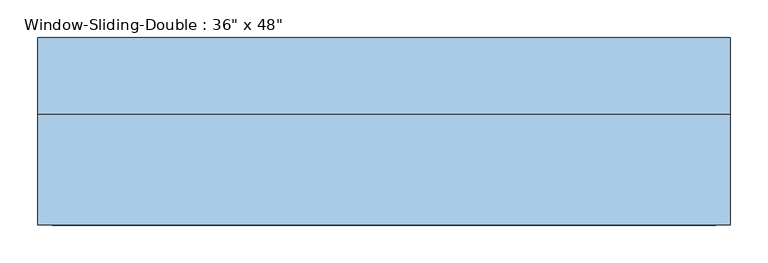
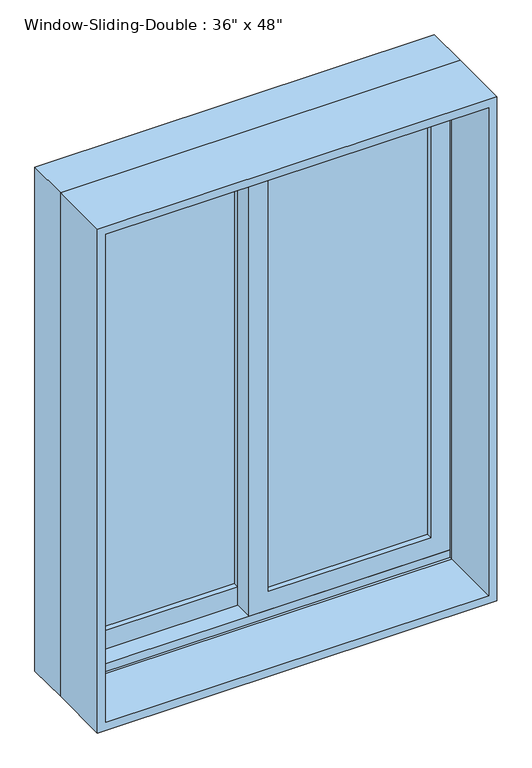
"""IFC4 building model written with IfcOpenShell, lengths in millimetres: window geometry."""

from ifc_helpers import new_model, si_unit, frame, origin, place, context, project, spatial, polyline, outline, extrude, faceted_brep, source, transform, mapped, element, save


def window_fdfe0ef3(model_context):
    return source(origin(), model_context, "Body", "SolidModel", [
        extrude(outline(polyline([(952.5, 438.15), (2114.55, 438.15), (2114.55, -22.225), (952.5, -22.225), (952.5, 438.15)]), holes=[polyline([(996.95, 22.225), (2070.1, 22.225), (2070.1, 393.7), (996.95, 393.7), (996.95, 22.225)])]), frame((0.0, 34.29, 0.0), z_axis=(0.0, 1.0, 0.0), x_axis=(0.0, 0.0, 1.0)), (0.0, 0.0, 1.0), 44.45),
        extrude(outline(polyline([(933.45, -438.15), (933.45, 22.225), (2114.55, 22.225), (2114.55, -438.15), (933.45, -438.15)]), holes=[polyline([(2070.1, -22.225), (996.95, -22.225), (996.95, -393.7), (2070.1, -393.7), (2070.1, -22.225)])]), frame((0.0, 78.74, 0.0), z_axis=(0.0, 1.0, 0.0), x_axis=(0.0, 0.0, 1.0)), (0.0, 0.0, 1.0), 44.45),
        extrude(outline(polyline([(-22.225, 110.49), (-22.225, 104.14), (-393.7, 104.14), (-393.7, 110.49), (-22.225, 110.49)])), frame((0.0, 0.0, 996.95), z_axis=(0.0, 0.0, 1.0), x_axis=(1.0, 0.0, 0.0)), (0.0, 0.0, 1.0), 1073.15),
        extrude(outline(polyline([(-22.225, 97.79), (-22.225, 91.44), (-393.7, 91.44), (-393.7, 97.79), (-22.225, 97.79)])), frame((0.0, 0.0, 996.95), z_axis=(0.0, 0.0, 1.0), x_axis=(1.0, 0.0, 0.0)), (0.0, 0.0, 1.0), 1073.15),
        extrude(outline(polyline([(393.7, 66.04), (393.7, 59.69), (22.225, 59.69), (22.225, 66.04), (393.7, 66.04)])), frame((0.0, 0.0, 996.95), z_axis=(0.0, 0.0, 1.0), x_axis=(1.0, 0.0, 0.0)), (0.0, 0.0, 1.0), 1073.15),
        extrude(outline(polyline([(393.7, 53.34), (393.7, 46.99), (22.225, 46.99), (22.225, 53.34), (393.7, 53.34)])), frame((0.0, 0.0, 996.95), z_axis=(0.0, 0.0, 1.0), x_axis=(1.0, 0.0, 0.0)), (0.0, 0.0, 1.0), 1073.15),
        extrude(outline(polyline([(2133.6, -457.2), (914.4, -457.2), (914.4, 457.2), (2133.6, 457.2), (2133.6, -457.2)]), holes=[polyline([(2114.55, 438.15), (933.45, 438.15), (933.45, -438.15), (2114.55, -438.15), (2114.55, 438.15)])]), frame((0.0, -118.11, 0.0), z_axis=(0.0, 1.0, 0.0), x_axis=(0.0, 0.0, 1.0)), (0.0, 0.0, 1.0), 146.05),
        faceted_brep([(-457.2, 27.94, 914.4), (-457.2, 129.54, 914.4), (457.2, 129.54, 914.4), (457.2, 27.94, 914.4), (-416.2778905, 129.54, 2092.6778905), (-416.2778905, 123.19, 2092.6778905), (-416.2778905, 123.19, 933.45), (-416.2778905, 129.54, 933.45), (416.2778905, 123.19, 2092.6778905), (416.2778905, 123.19, 933.45), (438.15, 123.19, 933.45), (438.15, 123.19, 2114.55), (-438.15, 123.19, 2114.55), (-438.15, 123.19, 933.45), (-438.15, 27.94, 2114.55), (-438.15, 27.94, 933.45), (-438.15, 34.29, 933.45), (-438.15, 34.29, 952.5), (-438.15, 78.74, 952.5), (-438.15, 78.74, 933.45), (457.2, 27.94, 2133.6), (-457.2, 27.94, 2133.6), (438.15, 27.94, 2114.55), (438.15, 27.94, 933.45), (-457.2, 129.54, 2133.6), (457.2, 129.54, 2133.6), (416.2778905, 129.54, 933.45), (416.2778905, 129.54, 2092.6778905), (438.15, 78.74, 933.45), (438.15, 78.74, 952.5), (438.15, 34.29, 952.5), (438.15, 34.29, 933.45)], [[[0, 1, 2, 3]], [[4, 5, 6, 7]], [[5, 8, 9, 10, 11, 12, 13, 6]], [[12, 14, 15, 16, 17, 18, 19, 13]], [[0, 3, 20, 21], [22, 23, 15, 14]], [[24, 1, 0, 21]], [[2, 1, 24, 25], [4, 7, 26, 27]], [[5, 4, 27, 8]], [[12, 11, 22, 14]], [[21, 20, 25, 24]], [[8, 27, 26, 9]], [[22, 11, 10, 28, 29, 30, 31, 23]], [[20, 3, 2, 25]], [[26, 7, 6, 13, 19, 28, 10, 9]], [[28, 19, 18, 29]], [[29, 18, 17, 30]], [[30, 17, 16, 31]], [[15, 23, 31, 16]]]),
    ])


if __name__ == "__main__":
    model = new_model("IFC4")
    model_context = context("Model", 3, world=origin())
    ifc_project = project(units=[si_unit("LENGTHUNIT", "METRE", prefix="MILLI")], contexts=[model_context])
    site = spatial("IfcSite", under=ifc_project)
    building = spatial("IfcBuilding", under=site)
    placement = place(None, origin())
    window_shape = window_fdfe0ef3(model_context)
    element("IfcWindow", 1, ObjectType="Window-Sliding-Double : 36\" x 48\"", at=placement, inside=building, context=model_context, shape_type="MappedRepresentation", body=[
        mapped(window_shape, transform((0.0, 0.0, 0.0), x_axis=(1.0, 0.0, 0.0), y_axis=(0.0, 1.0, 0.0), z_axis=(0.0, 0.0, 1.0))),
    ])
    save(model, "model.ifc")

# Revit data of these elements
# Type "Window-Sliding-Double : 36\" x 48\""
#   Type Mark = "23"
#   Fire Rating = "0.5h"
#   Analytic Construction = "Double glazing - domestic"
#   Window Inset [instance default] = 0' - 0"
#   Wall Thickness [instance default] = 0' - 6"
#   Visual Light Transmittance = 0.81
#   Thermal Resistance (R) = 1.8146 (h·ft²·°F)/BTU
#   Solar Heat Gain Coefficient = 0.76
#   Muntin Width = 1' - 2 5/8"
#   Muntin Height = 3' - 6 1/4"
#   Interior Wall Closure [instance default] = 0' - 2 3/4"
#   Heat Transfer Coefficient (U) = 0.5511 BTU/(h·ft²·°F)
#   Frame Extension [instance default] = 0' - 0 1/4"
#   Exterior Wall Closure [instance default] = 0' - 1 1/4"
#   Rough Width = 3' - 0 1/2"
#   Rough Height = 4' - 0 1/2"
#   Height = 4' - 0"
#   Extension Jamb [instance default] = 0' - 2 3/4"
#   Default Sill Height = 3' - 0"
#   Width = 3' - 0"
#   Interior Trim Visibility [instance default] = yes
#   Indicator Visibility [instance default] = yes
#   Exterior Trim Visibility [instance default] = yes
#   Muntin Visibility = yes
#   Extension Jamb Visibility [instance default] = yes
#   Muntin Pattern = Muntin Pattern_2x2 : Muntin Pattern_2x2
#   Interior Trim Material = Wood - Stained
#   Interior Trim = Trim-Window-Interior-Flat : Picture Frame
#   Interior Frame Material = Wood - Stained
#   Glass Panel Material = Glass
#   Exterior Trim Material = Clad - White
#   Exterior Trim = Trim-Window-Exterior-Flat : with Sill
#   Exterior Frame Material = Clad - White
#   Wall Closure = (empty or 0)
# Element 1 (IfcWindow, "Window-Sliding-Double : 36\" x 48\"")
#   Wall Thickness = 0' - 9"
#   Extension Jamb = 0' - 5 3/4"
#   Materials on its faces: "Wood - Stained", "Glass", "Clad - White"
# Materials
#   "Wood - Stained": class "Wood", colour RGB 224 178 126, transparency 0, Cost = 0
#   "Glass": class "Glass", colour RGB 0 128 192, transparency 0.75, Description = "Soda Lime Glass", Cost = 0
#   "Clad - White": class "Wood", colour RGB 242 242 238, transparency 0, Cost = 0
